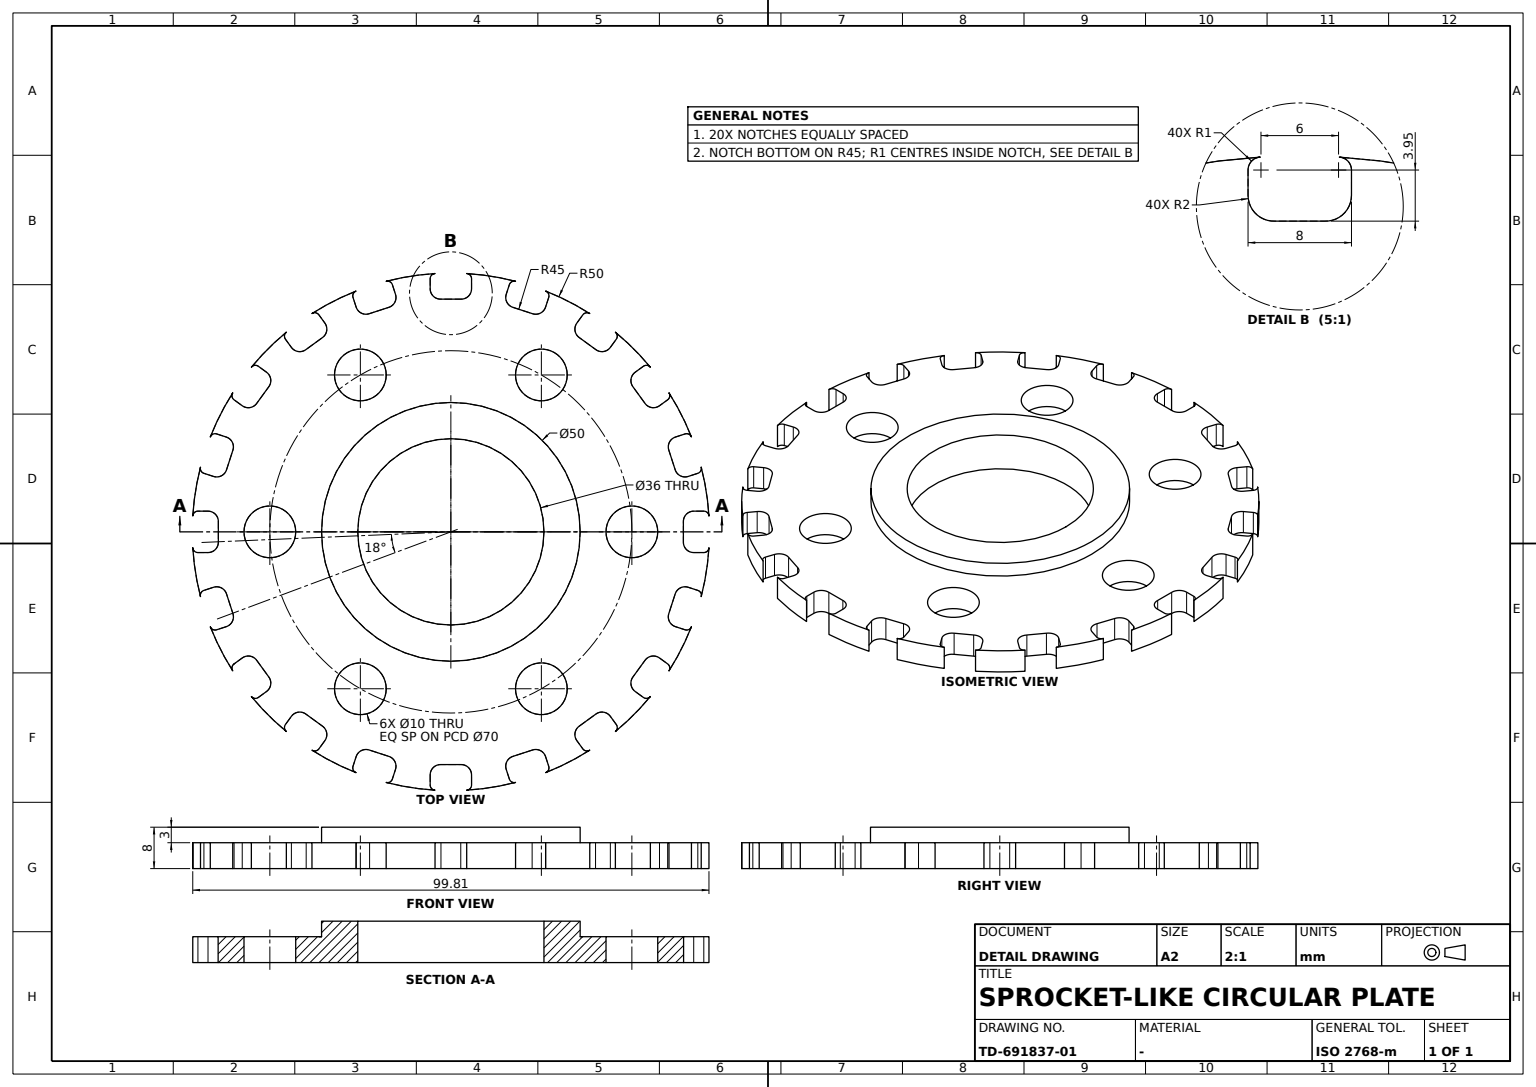
CATIA V5 part; units mm, degrees
sketch "Sketch1" plane through (0, 0, 0) normal (0, 0, 1) x (0, 1, 0)
  circle A0 centre (0, 0) radius 50
  dimension "radius A0" = 50
extrude "Pad1" add sketch "Sketch1" along normal mid plane 5
sketch "Sketch2" plane through (0, 0, 2.5) normal (0, 0, 1) x (0, 1, 0)
  arc A0 (1.9149, 44.9592) -> (-1.9149, 44.9592) centre (0, 0) ccw
  point P0 (4, 44.9206)
  point P1 (4, 48.9081)
  arc A1 (-1.9149, 44.9592) -> (-4, 46.9574) centre (-2, 46.9574) cw
  arc A2 (1.9149, 44.9592) -> (4, 46.9574) centre (2, 46.9574) ccw
  point P2 (4, 46.9574)
  line L0 (2.7594, 49.9238) -> (2.7594, 49.9238)
  line L1 (4, 48.9081) -> (4, 46.9574)
  point P3 (4, 48.9081)
  point P4 (4, 46.9574)
  circle A3 centre (0, 0) radius 50 construction
  arc A4 (3.0612, 49.9062) -> (-3.0612, 49.9062) centre (0, 0) ccw
  arc A5 (3.0612, 49.9062) -> (4, 48.9081) centre (3, 48.9081) cw
  point P5 (3.0612, 49.9062)
  point P6 (4, 48.9081)
  line L2 (-4, 46.9574) -> (-4, 48.9081)
  arc A6 (-3.0612, 49.9062) -> (-4, 48.9081) centre (-3, 48.9081) ccw
  point P7 (-3.0612, 49.9062)
  dimension "radius A0" = 45
  dimension "radius A1" = 2
  dimension "radius A2" = 2
  dimension "radius A5" = 1
  dimension "radius A6" = 1
  dimension "distance L2 L1" = 8
  constraint tangency A1 A0
  constraint tangency A2 A0
  constraint tangency A5 A3
  constraint tangency L2 A1
  constraint tangency A6 L2
  constraint tangency A6 A3
  constraint tangency A2 L1
  constraint tangency A5 L1
  constraint horizontal L0 x-axis
  constraint vertical L1 y-axis
  constraint coincidence P3 P1
  constraint coincidence P4 P2
  constraint coincidence A3 P5
  constraint coincidence P6 P1
  constraint coincidence A3 P7
  constraint symmetry L2 L1 y-axis
extrude "Pocket1" cut sketch "Sketch2" against normal through all
pattern_circular "CircPattern1" count 20 over 360 about axis through (0, 0, 0) along (0, 0, 1) of "Pocket1"
sketch "Sketch3" plane through (0, 0, 2.5) normal (0, 0, 1) x (0, 1, 0)
  circle A0 centre (0, 35) radius 5
  point P0 (0, 35)
  dimension "radius A0" = 5
  dimension "distance P0 x axis" = 35
  constraint coincidence P0 y-axis
extrude "Pocket2" cut sketch "Sketch3" against normal through all
pattern_circular "CircPattern2" count 6 over 360 about axis through (0, 0, 0) along (0, 0, 1) of "Pocket2"
sketch "Sketch4" plane through (0, 0, 2.5) normal (0, 0, 1) x (0, 1, 0)
  circle A0 centre (0, 0) radius 25
  dimension "radius A0" = 25
extrude "Pad2" add sketch "Sketch4" along normal blind 3
sketch "Sketch5" plane through (0, 0, 5.5) normal (0, 0, 1) x (0, 1, 0)
  circle A0 centre (0, 0) radius 18
  dimension "radius A0" = 18
extrude "Pocket3" cut sketch "Sketch5" against normal through all
equation "\"angular step@CircPattern1\" = 360.0*1 deg/CircPattern1.AngularNumber"
equation "\"angular step@CircPattern2\" = 360.0*1 deg/CircPattern2.AngularNumber"
